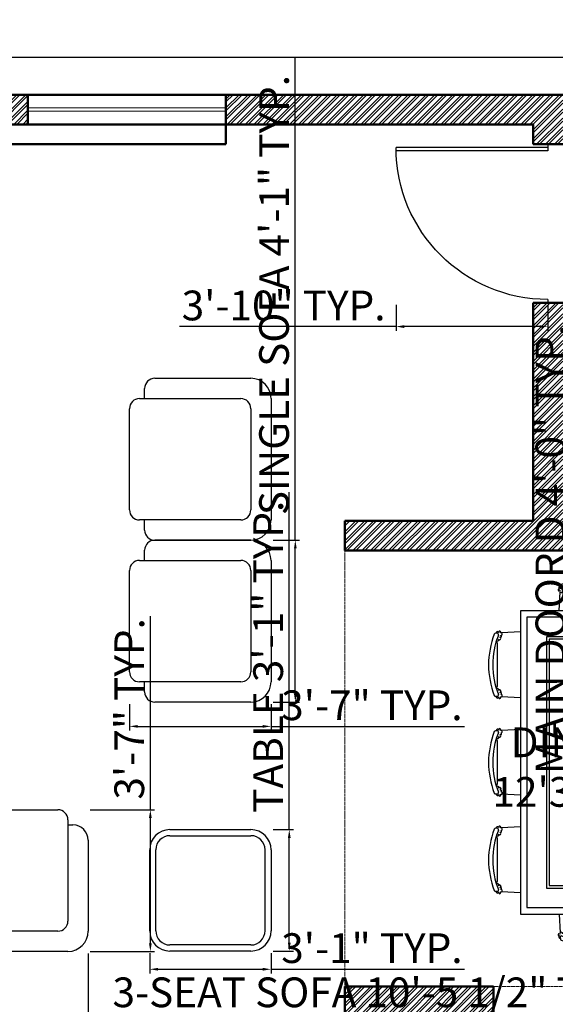
# Model space of a CAD drawing. Units: inches. Extents: x 3590 to 5167, y 65 to 1917.
# Tile 21 of 100: x 4051 to 4213, y 1531 to 1829. Entities that reach past the tile are written whole.
import ezdxf

# ---------------------------------------------------------------- set-up
doc = ezdxf.new("R2010")
doc.units = ezdxf.units.IN
doc.linetypes.add('DASHED', pattern=[0.75, 0.5, -0.25])
for name, color, linetype, lineweight in [('A-ANNO-DIMS', 2, 'Continuous', 18), ('A-AREA-IDEN', 7, 'Continuous', 18), ('A-DOOR', 3, 'Continuous', 25), ('A-FURN', 21, 'Continuous', 18), ('A-GLAZ', 4, 'Continuous', 18), ('A-WALL', 7, 'Continuous', 50), ('A-WALL-PATT', 251, 'Continuous', 13), ('S-BEAM-OVHD', 7, 'DASHED', 18)]:
    doc.layers.add(name, color=color, linetype=linetype, lineweight=lineweight)
for name, color, linetype in [('FUR', 42, 'Continuous'), ('HA', 9, 'Continuous'), ('M40-KOLTUKSUNGERI', 136, 'Continuous'), ('wood', 26, 'Continuous')]:
    doc.layers.add(name, color=color, linetype=linetype)
doc.styles.get("Standard").update_dxf_attribs({"font": 'arial.ttf'})
doc.dimstyles.new('ISO-25', dxfattribs={"dimtxt": 9, "dimasz": 2.5, "dimexe": 1.25, "dimexo": 0.625, "dimtad": 1, "dimdec": 1, "dimlunit": 3, "dimtxsty": 'Standard', "dimcen": 2.5, "dimadec": 0, "dimazin": 0, "dimtfac": 1, "dimtdec": 1, "dimtmove": 0, "dimatfit": 3, "dimfxl": 1, "dimarcsym": 0})

# ---------------------------------------------------------------- blocks, each defined once
blk = doc.blocks.new('*D5')
at = {"layer": 'A-ANNO-DIMS', "color": 0, "lineweight": -2, "transparency": 16777216}
for p, q in [((3645.51, 1806.62), (3645.51, 1818.61)), ((4305.51, 1806.62), (4305.51, 1818.61)), ((3648.01, 1817.36), (4303.01, 1817.36))]:
    blk.add_line(p, q, dxfattribs=at)
at = {"layer": 'A-ANNO-DIMS', "color": 0, "transparency": 16777216}
for points in [[(3648.01, 1817.78), (3648.01, 1816.95), (3645.51, 1817.36)], [(4303.01, 1817.78), (4303.01, 1816.95), (4305.51, 1817.36)]]:
    blk.add_solid(points, dxfattribs=at)
at = {"layer": 'Defpoints', "color": 0, "transparency": 16777216}
for p in [(4305.51, 1817.36), (3645.51, 1806), (4305.51, 1806)]:
    blk.add_point(p, dxfattribs=at)
at = {"layer": 'A-ANNO-DIMS', "color": 0, "transparency": 16777216, "insert": (3975.51, 1822.57), "char_height": 9, "attachment_point": 5}
blk.add_mtext("55'", dxfattribs=at)
blk = doc.blocks.new('D')
for p, q in [((1, 0), (1, 46)), ((2, 0), (2, 46)), ((0, 0), (2, 0)), ((47, 0), (48, 0))]:
    blk.add_line(p, q)
at = {"ltscale": 0.5}
blk.add_arc((1, 0), 46, 0, 90, dxfattribs=at)
blk = doc.blocks.new('S2')
at = {"layer": 'M40-KOLTUKSUNGERI'}
for p, q in [((-34.45, 27.56), (-14.76, 27.56)), ((-9.84, 27.56), (9.84, 27.56)), ((14.76, 27.56), (34.45, 27.56)), ((-36.42, 5.91), (-36.42, 25.59)), ((-12.8, 25.59), (-12.8, 5.91)), ((-11.81, 5.91), (-11.81, 25.59)), ((11.81, 25.59), (11.81, 5.91)), ((12.8, 5.91), (12.8, 25.59)), ((36.42, 25.59), (36.42, 5.91)), ((-37.4, 24.61), (-36.42, 24.61)), ((36.42, 24.61), (37.4, 24.61)), ((-40.35, 3.94), (-40.35, 21.65)), ((40.35, 21.65), (40.35, 3.94)), ((-14.76, 3.94), (-34.45, 3.94)), ((9.84, 3.94), (-9.84, 3.94)), ((34.45, 3.94), (14.76, 3.94)), ((36.42, 0), (-36.42, 0))]:
    blk.add_line(p, q, dxfattribs=at)
for centre, radius, start, end in [((-34.45, 25.59), 1.97, 90, 180), ((-14.76, 25.59), 1.97, 360, 90), ((-9.84, 25.59), 1.97, 90, 180), ((9.84, 25.59), 1.97, 360, 90), ((14.76, 25.59), 1.97, 90, 180), ((34.45, 25.59), 1.97, 360, 90), ((-37.4, 21.65), 2.95, 90, 180), ((37.4, 21.65), 2.95, 360, 90), ((-34.45, 5.91), 1.97, 180, 270), ((-14.76, 5.91), 1.97, 270, 0), ((-9.84, 5.91), 1.97, 180, 270), ((9.84, 5.91), 1.97, 270, 0), ((14.76, 5.91), 1.97, 180, 270), ((34.45, 5.91), 1.97, 270, 0), ((-36.42, 3.94), 3.94, 180, 270), ((36.42, 3.94), 3.94, 270, 0)]:
    blk.add_arc(centre, radius, start, end, dxfattribs=at)
blk = doc.blocks.new('S3')
at = {"layer": 'M40-KOLTUKSUNGERI'}
for p, q in [((-22.64, 15.75), (-3.94, 15.75)), ((-24.61, 11.81), (-24.61, 13.78)), ((-25.59, 11.81), (-5.91, 11.81)), ((0, 11.81), (0, -11.81)), ((-27.56, -9.84), (-27.56, 9.84)), ((-3.94, 9.84), (-3.94, -9.84)), ((-5.91, -11.81), (-25.59, -11.81)), ((-24.61, -13.78), (-24.61, -11.81)), ((-3.94, -15.75), (-22.64, -15.75))]:
    blk.add_line(p, q, dxfattribs=at)
for centre, radius, start, end in [((-22.64, 13.78), 1.97, 90, 180), ((-3.94, 11.81), 3.94, 360, 90), ((-25.59, 9.84), 1.97, 90, 180), ((-5.91, 9.84), 1.97, 360, 90), ((-25.59, -9.84), 1.97, 180, 270), ((-5.91, -9.84), 1.97, 270, 0), ((-3.94, -11.81), 3.94, 270, 0), ((-22.64, -13.78), 1.97, 180, 270)]:
    blk.add_arc(centre, radius, start, end, dxfattribs=at)
blk = doc.blocks.new('T2')
at = {"layer": 'M40-KOLTUKSUNGERI'}
for p, q in [((4874.89, 1687.13), (4890.64, 1687.13)), ((4874.89, 1685.95), (4890.64, 1685.95)), ((4870.95, 1667.45), (4870.95, 1683.2)), ((4872.13, 1667.45), (4872.13, 1683.2)), ((4893.39, 1683.2), (4893.39, 1667.45)), ((4894.57, 1683.2), (4894.57, 1667.45)), ((4890.64, 1664.69), (4874.89, 1664.69)), ((4890.64, 1663.51), (4874.89, 1663.51))]:
    blk.add_line(p, q, dxfattribs=at)
for centre, radius, start, end in [((4874.89, 1683.2), 3.94, 90, 180), ((4874.89, 1683.2), 2.76, 90, 180), ((4890.64, 1683.2), 3.94, 360, 90), ((4890.64, 1683.2), 2.76, 360, 90), ((4874.89, 1667.45), 3.94, 180, 270), ((4874.89, 1667.45), 2.76, 180, 270), ((4890.64, 1667.45), 3.94, 270, 0), ((4890.64, 1667.45), 2.76, 270, 0)]:
    blk.add_arc(centre, radius, start, end, dxfattribs=at)
blk = doc.blocks.new('A$C39F63D19')
at = {"layer": 'FUR'}
for p, q in [((1.415, 2.4468), (1.4061, 2.4547)), ((1.5486, 2.3264), (1.4408, 2.4235)), ((1.3599, 2.3864), (1.1308, 2.1573)), ((1.3599, 2.4017), (1.3588, 2.4028)), ((2.0077, 2.3522), (2.0166, 2.3602)), ((1.8741, 2.2319), (1.9819, 2.329)), ((2.0628, 2.3072), (2.0639, 2.3083)), ((2.0628, 2.2919), (2.2919, 2.0628)), ((1.1155, 2.1573), (1.1144, 2.1585)), ((1.1155, 2.1573), (1.1144, 2.1585)), ((1.0705, 2.1023), (1.0625, 2.1111)), ((1.1908, 1.9686), (1.0937, 2.0765)), ((2.3072, 2.0628), (2.3083, 2.0639)), ((2.3072, 2.0628), (2.3083, 2.0639)), ((2.2319, 1.8741), (2.329, 1.9819)), ((2.3522, 2.0077), (2.3602, 2.0166)), ((0.8846, 1.9165), (0.8758, 1.9244)), ((1.0183, 1.7961), (0.9104, 1.8932)), ((0.8296, 1.8561), (0.6005, 1.627)), ((0.8296, 1.8714), (0.8285, 1.8725)), ((0.5852, 1.627), (0.5841, 1.6281)), ((0.5852, 1.627), (0.5841, 1.6281)), ((0.5401, 1.572), (0.5322, 1.5808)), ((0.6605, 1.4383), (0.5634, 1.5462)), ((2.3264, 1.5486), (2.4235, 1.4408)), ((0.3543, 1.3861), (0.3455, 1.3941)), ((0.488, 1.2658), (0.3801, 1.3629)), ((2.4468, 1.415), (2.4547, 1.4061)), ((0.2993, 1.3258), (0.0701, 1.0967)), ((0.2993, 1.3411), (0.2981, 1.3422)), ((2.3864, 1.3599), (2.1573, 1.1308)), ((2.4017, 1.3599), (2.4028, 1.3588)), ((1.9686, 1.1908), (2.0765, 1.0937)), ((0.0549, 1.0967), (0.0538, 1.0978)), ((0.0549, 1.0967), (0.0538, 1.0978)), ((2.1023, 1.0705), (2.1111, 1.0625)), ((2.1573, 1.1155), (2.1585, 1.1144)), ((2.1573, 1.1155), (2.1585, 1.1144)), ((0.0098, 1.0416), (0.0019, 1.0505)), ((0.1302, 0.908), (0.033, 1.0158)), ((1.7961, 1.0183), (1.8932, 0.9104)), ((1.9165, 0.8846), (1.9244, 0.8758)), ((1.8561, 0.8296), (1.627, 0.6005)), ((1.8714, 0.8296), (1.8725, 0.8285)), ((1.4383, 0.6605), (1.5462, 0.5634)), ((0.2247, 0.5825), (0.1276, 0.4747)), ((1.572, 0.5401), (1.5808, 0.5322)), ((1.627, 0.5852), (1.6281, 0.5841)), ((1.627, 0.5852), (1.6281, 0.5841)), ((1.2658, 0.488), (1.3629, 0.3801)), ((0.1044, 0.4489), (0.0964, 0.44)), ((0.1494, 0.3938), (0.1483, 0.3927)), ((0.1647, 0.3938), (0.3938, 0.1647)), ((1.3861, 0.3543), (1.3941, 0.3455)), ((1.3258, 0.2993), (1.0967, 0.0701)), ((1.3411, 0.2993), (1.3422, 0.2981)), ((0.5825, 0.2247), (0.4747, 0.1276)), ((0.3938, 0.1494), (0.3927, 0.1483)), ((0.3938, 0.1494), (0.3927, 0.1483)), ((0.4489, 0.1044), (0.44, 0.0964)), ((0.908, 0.1302), (1.0158, 0.033)), ((1.0416, 0.0098), (1.0505, 0.0019)), ((1.0967, 0.0549), (1.0978, 0.0538)), ((1.0967, 0.0549), (1.0978, 0.0538))]:
    blk.add_line(p, q, dxfattribs=at)
for points in [[(1.6641, 2.4419), (0.0147, 0.7925), (0.7925, 0.0147), (2.4419, 1.6641)], [(1.6641, 2.3712), (0.0854, 0.7925), (0.7925, 0.0854), (2.3712, 1.6641)], [(1.6641, 2.159), (0.2976, 0.7925), (0.7925, 0.2976), (2.159, 1.6641)]]:
    blk.add_lwpolyline(points, close=True, dxfattribs=at)
for centre, radius, start, end in [((1.6574, 1.8598), 0.6521, 113.77302, 156.22698), ((1.6574, 1.8598), 0.6197, 113.33062, 156.66938), ((1.3989, 2.4467), 0.0108, 48, 113.77302), ((1.4185, 2.4458), 0.0101, 329.62103, 147.42526), ((1.4077, 2.4388), 0.0108, 293.33062, 48), ((1.4308, 2.4208), 0.0103, 213.3009, 71.36297), ((1.4349, 2.4385), 0.00795, 264.76881, 163.65384), ((1.3523, 2.3941), 0.0108, 315, 45), ((1.3814, 2.4068), 0.0085, 151.04971, 5.85435), ((1.3995, 2.4044), 0.0102, 161.25601, 35.99509), ((1.4156, 2.411), 0.00785, 184.4301, 31.81325), ((1.9878, 2.3439), 0.00795, 16.34616, 275.23119), ((2.0042, 2.3512), 0.0101, 32.57474, 210.37897), ((2.015, 2.3442), 0.0108, 132, 246.66938), ((2.0238, 2.3521), 0.0108, 66.22698, 132), ((1.7653, 1.7653), 0.6521, 23.77302, 66.22698), ((1.9919, 2.3262), 0.0103, 108.63703, 326.6991), ((2.0071, 2.3164), 0.00785, 148.18675, 355.5699), ((1.7653, 1.7653), 0.6197, 23.33062, 66.66938), ((2.0232, 2.3098), 0.0102, 144.00491, 18.74399), ((2.0413, 2.3122), 0.0085, 174.14565, 28.95029), ((2.0704, 2.2995), 0.0108, 135, 225), ((1.0705, 2.1184), 0.0108, 156.22698, 222), ((1.1105, 2.1359), 0.0085, 264.14565, 118.95029), ((1.1232, 2.165), 0.0108, 225, 315), ((1.0715, 2.0987), 0.0101, 122.57474, 300.37897), ((1.0785, 2.1095), 0.0108, 222, 336.66938), ((1.0788, 2.0824), 0.00795, 106.34616, 5.23119), ((1.0965, 2.0864), 0.0103, 198.63703, 56.6991), ((1.1063, 2.1017), 0.00785, 238.18675, 85.5699), ((2.2995, 2.0704), 0.0108, 225, 315), ((2.3122, 2.0413), 0.0085, 61.04971, 275.85435), ((2.3098, 2.0232), 0.0102, 71.25601, 305.99509), ((2.3164, 2.0071), 0.00785, 94.4301, 301.81325), ((2.3262, 1.9919), 0.0103, 123.3009, 341.36297), ((2.3442, 2.015), 0.0108, 203.33062, 318), ((2.3439, 1.9878), 0.00795, 174.76881, 73.65384), ((2.3512, 2.0042), 0.0101, 239.62103, 57.42526), ((2.3521, 2.0238), 0.0108, 318, 23.77302), ((1.1271, 1.3295), 0.6521, 113.77302, 156.22698), ((1.1271, 1.3295), 0.6197, 113.33062, 156.66938), ((0.8686, 1.9164), 0.0108, 48, 113.77302), ((0.8882, 1.9155), 0.0101, 329.62103, 147.42526), ((0.8774, 1.9084), 0.0108, 293.33062, 48), ((0.9005, 1.8904), 0.0103, 213.3009, 71.36297), ((0.9045, 1.9081), 0.00795, 264.76881, 163.65384), ((0.8219, 1.8638), 0.0108, 315, 45), ((0.8511, 1.8765), 0.0085, 151.04971, 5.85435), ((0.8692, 1.8741), 0.0102, 161.25601, 35.99509), ((0.8852, 1.8806), 0.00785, 184.4301, 31.81325), ((0.5402, 1.588), 0.0108, 156.22698, 222), ((0.5801, 1.6055), 0.0085, 264.14565, 118.95029), ((0.5825, 1.5874), 0.0102, 234.00491, 108.74399), ((0.5928, 1.6347), 0.0108, 225, 315), ((0.5411, 1.5684), 0.0101, 122.57474, 300.37897), ((0.5482, 1.5792), 0.0108, 222, 336.66938), ((0.5485, 1.5521), 0.00795, 106.34616, 5.23119), ((0.5662, 1.5561), 0.0103, 198.63703, 56.6991), ((0.576, 1.5714), 0.00785, 238.18675, 85.5699), ((2.4208, 1.4308), 0.0103, 18.63703, 236.6991), ((2.4385, 1.4349), 0.00795, 286.34616, 185.23119), ((0.5968, 0.7992), 0.6521, 113.77302, 156.22698), ((0.5968, 0.7992), 0.6197, 113.33062, 156.66938), ((0.3382, 1.3861), 0.0108, 48, 113.77302), ((0.3579, 1.3851), 0.0101, 329.62103, 147.42526), ((0.3471, 1.3781), 0.0108, 293.33062, 48), ((0.3702, 1.3601), 0.0103, 213.3009, 71.36297), ((0.3742, 1.3778), 0.00795, 264.76881, 163.65384), ((1.8598, 1.6574), 0.6197, 293.33062, 336.66938), ((1.8598, 1.6574), 0.6521, 293.77302, 336.22698), ((2.3941, 1.3523), 0.0108, 45, 135), ((2.4044, 1.3995), 0.0102, 54.00491, 288.74399), ((2.4068, 1.3814), 0.0085, 84.14565, 298.95029), ((2.411, 1.4156), 0.00785, 58.18675, 265.5699), ((2.4388, 1.4077), 0.0108, 42, 156.66938), ((2.4458, 1.4185), 0.0101, 302.57474, 120.37897), ((2.4467, 1.3989), 0.0108, 336.22698, 42), ((0.2916, 1.3334), 0.0108, 315, 45), ((0.3207, 1.3461), 0.0085, 151.04971, 5.85435), ((0.3388, 1.3437), 0.0102, 161.25601, 35.99509), ((0.3549, 1.3503), 0.00785, 184.4301, 31.81325), ((0.0099, 1.0577), 0.0108, 156.22698, 222), ((0.0498, 1.0752), 0.0085, 264.14565, 118.95029), ((0.0522, 1.0571), 0.0102, 234.00491, 108.74399), ((0.0625, 1.1043), 0.0108, 225, 315), ((2.0824, 1.0788), 0.00795, 84.76881, 343.65384), ((2.0864, 1.0965), 0.0103, 33.3009, 251.36297), ((2.0987, 1.0715), 0.0101, 149.62103, 327.42526), ((2.1017, 1.1063), 0.00785, 4.4301, 211.81325), ((2.1095, 1.0785), 0.0108, 113.33062, 228), ((2.1178, 1.1129), 0.0102, 341.25601, 215.99509), ((2.1184, 1.0705), 0.0108, 228, 293.77302), ((2.1359, 1.1105), 0.0085, 331.04971, 185.85435), ((2.165, 1.1232), 0.0108, 135, 225), ((0.0108, 1.0381), 0.0101, 122.57474, 300.37897), ((0.0178, 1.0489), 0.0108, 222, 336.66938), ((0.0181, 1.0217), 0.00795, 106.34616, 5.23119), ((0.0358, 1.0258), 0.0103, 198.63703, 56.6991), ((0.0456, 1.041), 0.00785, 238.18675, 85.5699), ((1.8904, 0.9005), 0.0103, 18.63703, 236.6991), ((1.9081, 0.9045), 0.00795, 286.34616, 185.23119), ((1.3295, 1.1271), 0.6197, 293.33062, 336.66938), ((1.3295, 1.1271), 0.6521, 293.77302, 336.22698), ((1.8741, 0.8692), 0.0102, 54.00491, 288.74399), ((1.8765, 0.8511), 0.0085, 84.14565, 298.95029), ((1.8806, 0.8852), 0.00785, 58.18675, 265.5699), ((1.9084, 0.8774), 0.0108, 42, 156.66938), ((1.9155, 0.8882), 0.0101, 302.57474, 120.37897), ((1.9164, 0.8686), 0.0108, 336.22698, 42), ((1.8638, 0.8219), 0.0108, 45, 135), ((1.5521, 0.5485), 0.00795, 84.76881, 343.65384), ((1.5561, 0.5662), 0.0103, 33.3009, 251.36297), ((1.5684, 0.5411), 0.0101, 149.62103, 327.42526), ((1.5714, 0.576), 0.00785, 4.4301, 211.81325), ((1.5792, 0.5482), 0.0108, 113.33062, 228), ((1.5874, 0.5825), 0.0102, 341.25601, 215.99509), ((1.588, 0.5402), 0.0108, 228, 293.77302), ((1.6055, 0.5801), 0.0085, 331.04971, 185.85435), ((1.6347, 0.5928), 0.0108, 135, 225), ((0.1054, 0.4524), 0.0101, 59.62103, 237.42526), ((0.1127, 0.4688), 0.00795, 354.76881, 253.65384), ((0.1304, 0.4647), 0.0103, 303.3009, 161.36297), ((0.1402, 0.4495), 0.00785, 274.4301, 121.81325), ((0.1044, 0.4328), 0.0108, 138, 203.77302), ((0.6913, 0.6913), 0.6521, 203.77302, 246.22698), ((0.1124, 0.4416), 0.0108, 23.33062, 138), ((0.6913, 0.6913), 0.6197, 203.33062, 246.66938), ((0.1444, 0.4153), 0.0085, 241.04971, 95.85435), ((0.1468, 0.4334), 0.0102, 251.25601, 125.99509), ((0.1571, 0.3862), 0.0108, 45, 135), ((1.3601, 0.3702), 0.0103, 18.63703, 236.6991), ((1.3778, 0.3742), 0.00795, 286.34616, 185.23119), ((0.7992, 0.5968), 0.6197, 293.33062, 336.66938), ((0.7992, 0.5968), 0.6521, 293.77302, 336.22698), ((1.3437, 0.3388), 0.0102, 54.00491, 288.74399), ((1.3461, 0.3207), 0.0085, 84.14565, 298.95029), ((1.3503, 0.3549), 0.00785, 58.18675, 265.5699), ((1.3781, 0.3471), 0.0108, 42, 156.66938), ((1.3851, 0.3579), 0.0101, 302.57474, 120.37897), ((1.3861, 0.3382), 0.0108, 336.22698, 42), ((1.3334, 0.2916), 0.0108, 45, 135), ((0.3862, 0.1571), 0.0108, 315, 45), ((0.4153, 0.1444), 0.0085, 354.14565, 208.95029), ((0.4334, 0.1468), 0.0102, 324.00491, 198.74399), ((0.4328, 0.1044), 0.0108, 246.22698, 312), ((0.4495, 0.1402), 0.00785, 328.18675, 175.5699), ((0.4524, 0.1054), 0.0101, 212.57474, 30.37897), ((0.4416, 0.1124), 0.0108, 312, 66.66938), ((0.4647, 0.1304), 0.0103, 288.63703, 146.6991), ((0.4688, 0.1127), 0.00795, 196.34616, 95.23119), ((1.0217, 0.0181), 0.00795, 84.76881, 343.65384), ((1.0258, 0.0358), 0.0103, 33.3009, 251.36297), ((1.0381, 0.0108), 0.0101, 149.62103, 327.42526), ((1.041, 0.0456), 0.00785, 4.4301, 211.81325), ((1.0489, 0.0178), 0.0108, 113.33062, 228), ((1.0571, 0.0522), 0.0102, 341.25601, 215.99509), ((1.0577, 0.0099), 0.0108, 228, 293.77302), ((1.0752, 0.0498), 0.0085, 331.04971, 185.85435), ((1.1043, 0.0625), 0.0108, 135, 225)]:
    blk.add_arc(centre, radius, start, end, dxfattribs=at)
at = {"layer": 'HA'}
blk.add_lwpolyline([(1.6641, 2.1308), (0.3258, 0.7925), (0.7925, 0.3258), (2.1308, 1.6641)], close=True, dxfattribs=at)
at = {"layer": 'wood'}
for points in [[(1.3825, 2.4152, 0.308332), (1.374, 2.4109, -0.00386)], [(1.4096, 2.4059, -0.15729), (1.4077, 2.4104, -0.120016)], [(1.1113, 2.1077, 1.044756), (1.1135, 2.1279, -0.117685), (1.1096, 2.1274, -1.643727), (1.1069, 2.1095, -0.15729)], [(2.3158, 2.015, -0.120016), (2.3113, 2.0131, -0.15729)], [(0.8522, 1.8849, 0.308332), (0.8436, 1.8806, -0.00386)], [(0.8792, 1.8756, -0.15729), (0.8774, 1.88, -0.120016)], [(0.581, 1.5774, 1.044756), (0.5832, 1.5976, -0.117685), (0.5793, 1.5971, -1.643727), (0.5766, 1.5792, -0.15729)], [(2.4104, 1.4077, -0.15729), (2.4059, 1.4096, 1.044756), (2.4037, 1.3893, -0.117685), (2.4077, 1.3899, -1.643727)], [(0.3489, 1.3453, -0.15729), (0.3471, 1.3497, -0.120016)], [(2.1095, 1.1069, -0.120016), (2.1077, 1.1113, -0.15729)], [(2.1347, 1.102, 0.308332), (2.1433, 1.1064, -0.00386)], [(1.88, 0.8774, -0.15729), (1.8756, 0.8792, 1.044756), (1.8734, 0.859, -0.117685), (1.8773, 0.8595, -1.643727)], [(1.5792, 0.5766, -0.120016), (1.5774, 0.581, -0.15729)], [(1.6044, 0.5717, 0.308332), (1.613, 0.576, -0.00386)], [(0.1453, 0.4435, -0.15729), (0.1408, 0.4416, -0.120016)], [(1.3497, 0.3471, -0.15729), (1.3453, 0.3489, 1.044756), (1.3431, 0.3287, -0.117685), (1.347, 0.3292, -1.643727)], [(1.0489, 0.0462, -0.120016), (1.047, 0.0507, -0.15729)], [(1.0741, 0.0414, 0.308332), (1.0826, 0.0457, -0.00386)]]:
    blk.add_lwpolyline(points, format="xyb", close=True, dxfattribs=at)
blk = doc.blocks.new('*D294')
at = {"layer": 'A-ANNO-DIMS', "color": 0, "lineweight": -2, "transparency": 16777216}
for p, q in [((3946.19, 1546.03), (3946.19, 1526.56)), ((4071.76, 1546.03), (4071.76, 1526.56)), ((3948.69, 1527.81), (4069.26, 1527.81)), ((4071.76, 1527.81), (4243.57, 1527.81))]:
    blk.add_line(p, q, dxfattribs=at)
at = {"layer": 'A-ANNO-DIMS', "color": 0, "transparency": 16777216}
for points in [[(3948.69, 1528.23), (3948.69, 1527.4), (3946.19, 1527.81)], [(4069.26, 1528.23), (4069.26, 1527.4), (4071.76, 1527.81)]]:
    blk.add_solid(points, dxfattribs=at)
at = {"layer": 'Defpoints', "color": 0, "transparency": 16777216}
for p in [(3946.19, 1546.65), (4071.76, 1546.65), (4071.76, 1527.81)]:
    blk.add_point(p, dxfattribs=at)
at = {"layer": 'A-ANNO-DIMS', "color": 0, "transparency": 16777216, "insert": (4158.91, 1533.1), "char_height": 9, "attachment_point": 5}
blk.add_mtext('3-SEAT SOFA 10\'-5 1/2" TYP.', dxfattribs=at)
blk = doc.blocks.new('*D295')
at = {"layer": 'A-ANNO-DIMS', "color": 0, "lineweight": -2, "transparency": 16777216}
for p, q in [((4090.6, 1589.53), (4090.6, 1648.13)), ((4072.39, 1589.53), (4091.85, 1589.53)), ((4090.6, 1549.15), (4090.6, 1587.03)), ((4072.39, 1546.65), (4091.85, 1546.65))]:
    blk.add_line(p, q, dxfattribs=at)
at = {"layer": 'A-ANNO-DIMS', "color": 0, "transparency": 16777216}
for points in [[(4090.18, 1587.03), (4091.02, 1587.03), (4090.6, 1589.53)], [(4090.18, 1549.15), (4091.02, 1549.15), (4090.6, 1546.65)]]:
    blk.add_solid(points, dxfattribs=at)
at = {"layer": 'Defpoints', "color": 0, "transparency": 16777216}
for p in [(4071.76, 1589.53), (4090.6, 1589.53), (4071.76, 1546.65)]:
    blk.add_point(p, dxfattribs=at)
at = {"layer": 'A-ANNO-DIMS', "color": 0, "transparency": 16777216, "insert": (4085.38, 1620.08), "char_height": 9, "attachment_point": 5, "rotation": 90}
blk.add_mtext('3\'-7" TYP.', dxfattribs=at)
blk = doc.blocks.new('*D296')
at = {"layer": 'A-ANNO-DIMS', "color": 0, "lineweight": -2, "transparency": 16777216}
for p, q in [((4134.51, 1671.13), (4134.51, 1817.03)), ((4127.79, 1671.13), (4135.76, 1671.13)), ((4134.51, 1624.63), (4134.51, 1668.63)), ((4127.79, 1622.13), (4135.76, 1622.13))]:
    blk.add_line(p, q, dxfattribs=at)
at = {"layer": 'A-ANNO-DIMS', "color": 0, "transparency": 16777216}
for points in [[(4134.1, 1668.63), (4134.93, 1668.63), (4134.51, 1671.13)], [(4134.1, 1624.63), (4134.93, 1624.63), (4134.51, 1622.13)]]:
    blk.add_solid(points, dxfattribs=at)
at = {"layer": 'Defpoints', "color": 0, "transparency": 16777216}
for p in [(4127.16, 1671.13), (4134.51, 1671.13), (4127.16, 1622.13)]:
    blk.add_point(p, dxfattribs=at)
at = {"layer": 'A-ANNO-DIMS', "color": 0, "transparency": 16777216, "insert": (4129.23, 1745.33), "char_height": 9, "attachment_point": 5, "rotation": 90}
blk.add_mtext('SINGLE SOFA 4\'-1" TYP.', dxfattribs=at)
blk = doc.blocks.new('*D297')
at = {"layer": 'A-ANNO-DIMS', "color": 0, "lineweight": -2, "transparency": 16777216}
for p, q in [((4084.28, 1621.5), (4084.28, 1613.53)), ((4127.16, 1621.5), (4127.16, 1613.53)), ((4086.78, 1614.78), (4124.66, 1614.78)), ((4127.16, 1614.78), (4185.77, 1614.78))]:
    blk.add_line(p, q, dxfattribs=at)
at = {"layer": 'A-ANNO-DIMS', "color": 0, "transparency": 16777216}
for points in [[(4086.78, 1615.19), (4086.78, 1614.36), (4084.28, 1614.78)], [(4124.66, 1615.19), (4124.66, 1614.36), (4127.16, 1614.78)]]:
    blk.add_solid(points, dxfattribs=at)
at = {"layer": 'Defpoints', "color": 0, "transparency": 16777216}
for p in [(4084.28, 1622.13), (4127.16, 1622.13), (4127.16, 1614.78)]:
    blk.add_point(p, dxfattribs=at)
at = {"layer": 'A-ANNO-DIMS', "color": 0, "transparency": 16777216, "insert": (4157.71, 1620), "char_height": 9, "attachment_point": 5}
blk.add_mtext('3\'-7" TYP.', dxfattribs=at)
blk = doc.blocks.new('*D300')
at = {"layer": 'A-ANNO-DIMS', "color": 0, "lineweight": -2, "transparency": 16777216}
for p, q in [((4132.68, 1583.52), (4132.68, 1685.68)), ((4127.79, 1583.52), (4133.93, 1583.52)), ((4132.68, 1549.27), (4132.68, 1581.02)), ((4127.79, 1546.77), (4133.93, 1546.77))]:
    blk.add_line(p, q, dxfattribs=at)
at = {"layer": 'A-ANNO-DIMS', "color": 0, "transparency": 16777216}
for points in [[(4132.26, 1581.02), (4133.09, 1581.02), (4132.68, 1583.52)], [(4132.26, 1549.27), (4133.09, 1549.27), (4132.68, 1546.77)]]:
    blk.add_solid(points, dxfattribs=at)
at = {"layer": 'Defpoints', "color": 0, "transparency": 16777216}
for p in [(4127.16, 1583.52), (4132.68, 1583.52), (4127.16, 1546.77)]:
    blk.add_point(p, dxfattribs=at)
at = {"layer": 'A-ANNO-DIMS', "color": 0, "transparency": 16777216, "insert": (4127.45, 1635.85), "char_height": 9, "attachment_point": 5, "rotation": 90}
blk.add_mtext('TABLE 3\'-1" TYP.', dxfattribs=at)
blk = doc.blocks.new('*D301')
at = {"layer": 'A-ANNO-DIMS', "color": 0, "lineweight": -2, "transparency": 16777216}
for p, q in [((4090.41, 1546.14), (4090.41, 1540)), ((4127.16, 1546.14), (4127.16, 1540)), ((4092.91, 1541.25), (4124.66, 1541.25)), ((4127.16, 1541.25), (4185.77, 1541.25))]:
    blk.add_line(p, q, dxfattribs=at)
at = {"layer": 'A-ANNO-DIMS', "color": 0, "transparency": 16777216}
for points in [[(4092.91, 1541.67), (4092.91, 1540.84), (4090.41, 1541.25)], [(4124.66, 1541.67), (4124.66, 1540.84), (4127.16, 1541.25)]]:
    blk.add_solid(points, dxfattribs=at)
at = {"layer": 'Defpoints', "color": 0, "transparency": 16777216}
for p in [(4090.41, 1546.77), (4127.16, 1546.77), (4127.16, 1541.25)]:
    blk.add_point(p, dxfattribs=at)
at = {"layer": 'A-ANNO-DIMS', "color": 0, "transparency": 16777216, "insert": (4157.71, 1546.48), "char_height": 9, "attachment_point": 5}
blk.add_mtext('3\'-1" TYP.', dxfattribs=at)
blk = doc.blocks.new('*D316')
at = {"layer": 'A-ANNO-DIMS', "color": 0, "lineweight": -2, "transparency": 16777216}
for p, q in [((4211.64, 1791), (4219.46, 1791)), ((4218.21, 1788.5), (4218.21, 1745.5)), ((4211.64, 1743), (4219.46, 1743)), ((4218.21, 1743), (4218.21, 1596.09))]:
    blk.add_line(p, q, dxfattribs=at)
at = {"layer": 'A-ANNO-DIMS', "color": 0, "transparency": 16777216}
for points in [[(4217.8, 1788.5), (4218.63, 1788.5), (4218.21, 1791)], [(4217.8, 1745.5), (4218.63, 1745.5), (4218.21, 1743)]]:
    blk.add_solid(points, dxfattribs=at)
at = {"layer": 'Defpoints', "color": 0, "transparency": 16777216}
for p in [(4211.01, 1791), (4211.01, 1743), (4218.21, 1743)]:
    blk.add_point(p, dxfattribs=at)
at = {"layer": 'A-ANNO-DIMS', "color": 0, "transparency": 16777216, "insert": (4212.93, 1668.29), "char_height": 9, "attachment_point": 5, "rotation": 90}
blk.add_mtext('MAIN DOOR D 4\'-0" TYP.', dxfattribs=at)
blk = doc.blocks.new('*D317')
at = {"layer": 'A-ANNO-DIMS', "color": 0, "lineweight": -2, "transparency": 16777216}
for p, q in [((4165.01, 1742.37), (4165.01, 1734.55)), ((4211.01, 1742.37), (4211.01, 1734.55)), ((4165.01, 1735.8), (4099.42, 1735.8)), ((4208.51, 1735.8), (4167.51, 1735.8))]:
    blk.add_line(p, q, dxfattribs=at)
at = {"layer": 'A-ANNO-DIMS', "color": 0, "transparency": 16777216}
for points in [[(4167.51, 1736.22), (4167.51, 1735.38), (4165.01, 1735.8)], [(4208.51, 1736.22), (4208.51, 1735.38), (4211.01, 1735.8)]]:
    blk.add_solid(points, dxfattribs=at)
at = {"layer": 'Defpoints', "color": 0, "transparency": 16777216}
for p in [(4165.01, 1743), (4211.01, 1743), (4165.01, 1735.8)]:
    blk.add_point(p, dxfattribs=at)
at = {"layer": 'A-ANNO-DIMS', "color": 0, "transparency": 16777216, "insert": (4130.96, 1741.02), "char_height": 9, "attachment_point": 5}
blk.add_mtext('3\'-10" TYP.', dxfattribs=at)

msp = doc.modelspace()

# ---------------------------------------------------------------- hatches: boundary and pattern name
at = {"layer": 'A-WALL-PATT', "transparency": 33554687}
h = msp.add_hatch(dxfattribs=at)
h.set_pattern_fill('ANSI32', color=256, scale=0.2)
h.paths.add_polyline_path([(3768.51, 1806), (3645.51, 1806), (3645.51, 1785), (3654.51, 1785), (3654.51, 1797), (3671.16, 1797), (3768.51, 1797)])
h.paths.add_polyline_path([(3909.51, 1806), (3816.51, 1806), (3816.51, 1797), (3864.51, 1797), (3864.51, 1791), (3873.51, 1791), (3873.51, 1797), (3909.51, 1797)])
h.paths.add_polyline_path([(4053.51, 1806), (3969.51, 1806), (3969.51, 1797), (4053.51, 1797)])
h.paths.add_polyline_path([(4215.51, 1806), (4113.51, 1806), (4113.51, 1797), (4206.51, 1797), (4206.51, 1791), (4215.51, 1791)])
h.paths.add_polyline_path([(3654.51, 1737), (3645.51, 1737), (3645.51, 1620), (3654.51, 1620), (3654.51, 1650), (3741.51, 1650), (3741.51, 1656), (3654.51, 1656)], flags=17)
h.paths.add_polyline_path([(3873.51, 1755), (3864.51, 1755), (3864.51, 1656), (3771.51, 1656), (3771.51, 1650), (3774.51, 1650), (3774.51, 1554), (3654.51, 1554), (3654.51, 1584), (3645.51, 1584), (3645.51, 1539), (3654.51, 1539), (3654.51, 1545), (3864.51, 1545), (3864.51, 1539), (3873.51, 1539), (3873.51, 1584), (3864.51, 1584), (3864.51, 1554), (3780.51, 1554), (3780.51, 1650), (3864.51, 1650), (3864.51, 1620), (3873.51, 1620)])
h.paths.add_polyline_path([(3654.51, 1491), (3645.51, 1491), (3645.51, 1326), (3810.51, 1326), (3810.51, 1335), (3809.96, 1335), (3654.51, 1335)])
h.paths.add_polyline_path([(3915.51, 1335), (3873.51, 1335), (3873.51, 1352.87), (3873.51, 1422), (3876.51, 1422), (3876.51, 1431), (3864.51, 1431), (3864.51, 1335), (3858.51, 1335), (3858.51, 1326), (3915.51, 1326)])
h.paths.add_polyline_path([(4028.01, 1335), (4002.51, 1335), (4002.51, 1503), (3981.51, 1503), (3981.51, 1494), (3993.51, 1494), (3993.51, 1431), (3921.51, 1431), (3921.51, 1494), (3933.51, 1494), (3933.51, 1503), (3864.51, 1503), (3864.51, 1494), (3912.51, 1494), (3912.51, 1431), (3906.51, 1431), (3906.51, 1422), (3993.51, 1422), (3993.51, 1335), (3951.51, 1335), (3951.51, 1326), (4028.01, 1326)])
h.paths.add_polyline_path([(4203.51, 1335), (4158.51, 1335), (4158.51, 1527), (4194.51, 1527), (4194.51, 1536), (4149.51, 1536), (4149.51, 1335), (4124.01, 1335), (4124.01, 1326), (4203.51, 1326)])
h.paths.add_polyline_path([(4305.51, 1566), (4296.51, 1566), (4296.51, 1536), (4278.64, 1536), (4260.51, 1536), (4260.51, 1527), (4296.51, 1527), (4296.51, 1521), (4305.51, 1521)])
h.paths.add_polyline_path([(4305.51, 1473), (4296.51, 1473), (4296.51, 1335), (4251.51, 1335), (4251.51, 1326), (4305.51, 1326)])
h.paths.add_polyline_path([(4305.51, 1677), (4215.51, 1677), (4215.51, 1743), (4206.51, 1743), (4206.51, 1677), (4149.51, 1677), (4149.51, 1668), (4296.51, 1668), (4296.51, 1638), (4305.51, 1638)])

# ---------------------------------------------------------------- linework, layer by layer
at = {"layer": 'A-GLAZ'}
for p, q in [((4113.51, 1802), (4053.51, 1802)), ((4113.51, 1801), (4053.51, 1801))]:
    msp.add_line(p, q, dxfattribs=at)
at = {"layer": 'A-WALL'}
for p, q in [((4053.51, 1797), (4053.51, 1806)), ((4113.51, 1797), (4113.51, 1806)), ((3873.51, 1797), (4206.51, 1797)), ((4113.51, 1797), (4113.51, 1791)), ((4206.51, 1797), (4206.51, 1791)), ((4041.51, 1791), (4113.51, 1791)), ((4206.51, 1791), (4215.51, 1791)), ((4206.51, 1743), (4215.51, 1743)), ((4206.51, 1743), (4206.51, 1677)), ((4149.51, 1668), (4149.51, 1677)), ((4206.51, 1677), (4149.51, 1677)), ((4296.51, 1668), (4149.51, 1668)), ((4149.51, 1335), (4149.51, 1536)), ((4194.51, 1536), (4149.51, 1536)), ((4194.51, 1527), (4194.51, 1536))]:
    msp.add_line(p, q, dxfattribs=at)
msp.add_lwpolyline([(4305.51, 1677), (4305.51, 1326), (3645.51, 1326), (3645.51, 1806), (4215.51, 1806)], dxfattribs=at)
at = {"layer": 'S-BEAM-OVHD', "ltscale": 0.5}
for p, q in [((4149.51, 1668), (4149.51, 1536)), ((4194.51, 1536), (4260.51, 1536))]:
    msp.add_line(p, q, dxfattribs=at)

# ---------------------------------------------------------------- block references
at = {"layer": 'A-DOOR', "xscale": -1, "rotation": 90}
msp.add_blockref('D', (4211.01, 1791), dxfattribs=at)
at = {"layer": 'A-FURN', "xscale": 1.555868517605225, "yscale": 1.555868517605225, "zscale": 1.555868517605225}
for name, p in [('S3', (4127.16, 1695.63)), ('S3', (4127.16, 1646.63)), ('S2', (4008.98, 1546.65)), ('T2', (-3488.15, -1041.44))]:
    msp.add_blockref(name, p, dxfattribs=at)
at = {"layer": 'A-FURN', "xscale": 39.3701, "yscale": 39.3701, "zscale": 39.3701, "rotation": 225.0000000000003}
msp.add_blockref('A$C39F63D19', (4224.35, 1672.27), dxfattribs=at)

# ---------------------------------------------------------------- texts
at = {"layer": 'A-AREA-IDEN', "insert": (4194.24, 1614.45), "char_height": 9, "attachment_point": 1}
msp.add_mtext_dynamic_manual_height_columns('{\\fTimes New Roman|b0|i0|c0|p18;  DINING\\P12\'3"X11\'0"}', width=67.3508, gutter_width=12.5, heights=[0], dxfattribs=at)

# ---------------------------------------------------------------- dimensions: what is measured, and where the dimension line sits
at = {"layer": 'A-ANNO-DIMS'}
dim = msp.add_linear_dim(base=(4305.51, 1817.36), p1=(3645.51, 1806), p2=(4305.51, 1806), dimstyle='ISO-25', override={"dimclrd": 0, "dimclre": 0, "dimclrt": 0}, dxfattribs=at)
dim.commit()
dim.dimension.update_dxf_attribs({"geometry": '*D5', "text_midpoint": (3975.51, 1822.57)})
for base, p1, p2, angle, text, picture, middle in [((4134.51, 1671.13), (4127.16, 1622.13), (4127.16, 1671.13), 90, 'SINGLE SOFA <> TYP.', '*D296', (4129.23, 1745.33)), ((4218.21, 1743), (4211.01, 1791), (4211.01, 1743), 270, 'MAIN DOOR D <> TYP.', '*D316', (4212.93, 1668.29)), ((4165.01, 1735.8), (4211.01, 1743), (4165.01, 1743), 180, '<> TYP.', '*D317', (4130.96, 1741.02)), ((4132.6754, 1583.5207), (4127.1624, 1546.7679), (4127.1624, 1583.5207), 90, 'TABLE <> TYP.', '*D300', (4127.4521, 1635.851)), ((4090.6, 1589.53), (4071.76, 1546.65), (4071.76, 1589.53), 90, '<> TYP.', '*D295', (4085.38, 1620.08))]:
    dim = msp.add_linear_dim(base=base, p1=p1, p2=p2, angle=angle, text=text, dimstyle='ISO-25', override={"dimdec": 1, "dimlfac": 1, "dimrnd": 0, "dimzin": 1, "dimdsep": 46, "dimlunit": 4, "dimfrac": 2}, dxfattribs=at)
    dim.commit()
    dim.dimension.update_dxf_attribs({"geometry": picture, "text_midpoint": middle})
for base, p1, p2, text, picture, middle in [((4127.16, 1614.78), (4084.28, 1622.13), (4127.16, 1622.13), '<> TYP.', '*D297', (4157.71, 1620)), ((4071.76, 1527.81), (3946.19, 1546.65), (4071.76, 1546.65), '3-SEAT SOFA <> TYP.', '*D294', (4158.91, 1533.1)), ((4127.1624, 1541.255), (4090.4096, 1546.7679), (4127.1624, 1546.7679), '<> TYP.', '*D301', (4157.7141, 1546.4782))]:
    dim = msp.add_linear_dim(base=base, p1=p1, p2=p2, text=text, dimstyle='ISO-25', override={"dimdec": 1, "dimlfac": 1, "dimrnd": 0, "dimzin": 1, "dimdsep": 46, "dimlunit": 4, "dimfrac": 2}, dxfattribs=at)
    dim.commit()
    dim.dimension.update_dxf_attribs({"geometry": picture, "text_midpoint": middle})

doc.saveas('drawing.dxf')
